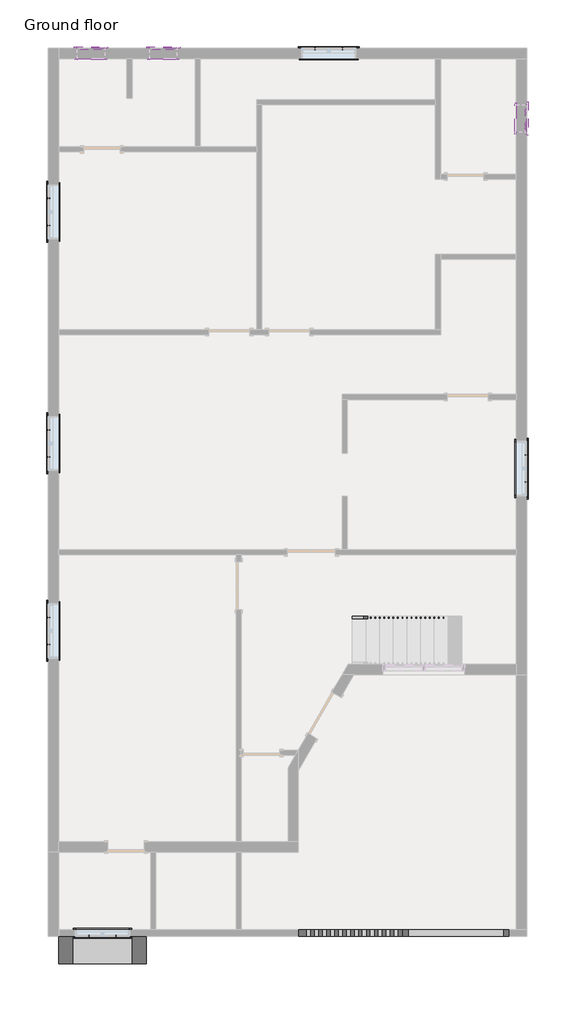
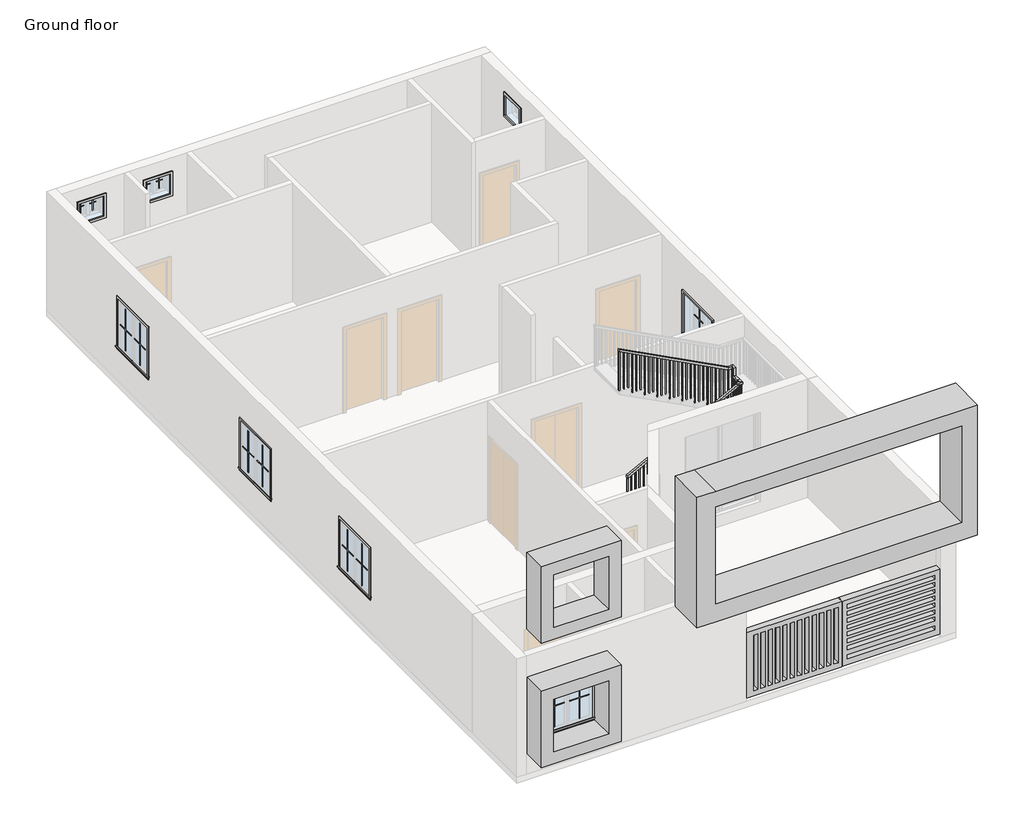
# One storey, part 3 of 3: 37 proxies, 1 railing.
"""IFC4 building model written with IfcOpenShell, lengths in millimetres."""

from ifc_helpers import new_model, si_unit, frame, origin, place, context, project, spatial, polyline, outline, extrude, faceted_brep, transform, mapped, element, save
from components import generic_models_1_generic_models_1_e6b78f1d, muntin_pattern_2x2_muntin_pattern_2x2_4dfeb3f3, muntin_pattern_2x2_muntin_pattern_2x2_e852a7e4, muntin_pattern_2x2_muntin_pattern_2x2_653c8599, muntin_pattern_2x2_muntin_pattern_2x2_c179cf80, trim_window_exterior_flat_with_sill_7cfdd449, trim_window_exterior_flat_with_sill_e6f34eb5, trim_window_interior_flat_picture_frame_f1e0b15b, trim_window_interior_flat_picture_frame_9a74d23d

model = new_model("IFC4")

# Units and contexts
model_context = context("Model", 3, world=origin())
ifc_project = project(units=[si_unit("LENGTHUNIT", "METRE", prefix="MILLI")], contexts=[model_context])

# Site, building, storey
site = spatial("IfcSite", under=ifc_project)
building = spatial("IfcBuilding", under=site)
storey = spatial("IfcBuildingStorey", under=building, Name="Ground floor", Elevation=0.0)

# Proxies
placement = place(None, origin())
generic_models_1_generic_models_1_shape = generic_models_1_generic_models_1_e6b78f1d(model_context)
element("IfcBuildingElementProxy", 1, Name="Generic Models 1 : Generic Models 1", ObjectType="Generic Models 1 : Generic Models 1", at=placement, inside=storey, context=model_context, shape_type="MappedRepresentation", body=[
    mapped(generic_models_1_generic_models_1_shape, transform((0.0, 0.0, 0.0), x_axis=(1.0, 0.0, 0.0), y_axis=(0.0, 1.0, 0.0), z_axis=(0.0, 0.0, 1.0))),
])
muntin_pattern_2x2_muntin_pattern_2x2_shape = muntin_pattern_2x2_muntin_pattern_2x2_4dfeb3f3(model_context)
element("IfcBuildingElementProxy", 2, Name="Muntin Pattern_2x2 : Muntin Pattern_2x2", ObjectType="Muntin Pattern_2x2 : Muntin Pattern_2x2", at=placement, inside=storey, context=model_context, shape_type="MappedRepresentation", body=[
    mapped(muntin_pattern_2x2_muntin_pattern_2x2_shape, transform((-5762.6039904, 6205.1114079, 984.25), x_axis=(0.0, 1.0, 0.0), y_axis=(-1.0, 0.0, 0.0), z_axis=(0.0, 0.0, 1.0))),
])
element("IfcBuildingElementProxy", 3, Name="Muntin Pattern_2x2 : Muntin Pattern_2x2", ObjectType="Muntin Pattern_2x2 : Muntin Pattern_2x2", at=placement, inside=storey, context=model_context, shape_type="MappedRepresentation", body=[
    mapped(muntin_pattern_2x2_muntin_pattern_2x2_shape, transform((-5762.6039904, 1040.9857391, 984.25), x_axis=(0.0, 1.0, 0.0), y_axis=(-1.0, 0.0, 0.0), z_axis=(0.0, 0.0, 1.0))),
])
element("IfcBuildingElementProxy", 4, Name="Muntin Pattern_2x2 : Muntin Pattern_2x2", ObjectType="Muntin Pattern_2x2 : Muntin Pattern_2x2", at=placement, inside=storey, context=model_context, shape_type="MappedRepresentation", body=[
    mapped(muntin_pattern_2x2_muntin_pattern_2x2_shape, transform((-5762.6039904, -3142.7752914, 984.25), x_axis=(0.0, 1.0, 0.0), y_axis=(-1.0, 0.0, 0.0), z_axis=(0.0, 0.0, 1.0))),
])
element("IfcBuildingElementProxy", 5, Name="Muntin Pattern_2x2 : Muntin Pattern_2x2", ObjectType="Muntin Pattern_2x2 : Muntin Pattern_2x2", at=placement, inside=storey, context=model_context, shape_type="MappedRepresentation", body=[
    mapped(muntin_pattern_2x2_muntin_pattern_2x2_shape, transform((4887.9335096, 1085.6654692, 984.25), x_axis=(0.0, -1.0, 0.0), y_axis=(1.0, 0.0, 0.0), z_axis=(0.0, 0.0, 1.0))),
])
element("IfcBuildingElementProxy", 6, Name="Muntin Pattern_2x2 : Muntin Pattern_2x2", ObjectType="Muntin Pattern_2x2 : Muntin Pattern_2x2", at=placement, inside=storey, context=model_context, shape_type="MappedRepresentation", body=[
    mapped(muntin_pattern_2x2_muntin_pattern_2x2_shape, transform((-4258.4477404, -9644.6273906, 984.25), x_axis=(-1.0, 0.0, 0.0), y_axis=(0.0, -1.0, 0.0), z_axis=(0.0, 0.0, 1.0))),
])
element("IfcBuildingElementProxy", 7, Name="Muntin Pattern_2x2 : Muntin Pattern_2x2", ObjectType="Muntin Pattern_2x2 : Muntin Pattern_2x2", at=placement, inside=storey, context=model_context, shape_type="MappedRepresentation", body=[
    mapped(muntin_pattern_2x2_muntin_pattern_2x2_shape, transform((180.9960096, 10148.3226094, 984.25), x_axis=(1.0, 0.0, 0.0), y_axis=(0.0, 1.0, 0.0), z_axis=(0.0, 0.0, 1.0))),
])
muntin_pattern_2x2_muntin_pattern_2x2_2_shape = muntin_pattern_2x2_muntin_pattern_2x2_e852a7e4(model_context)
element("IfcBuildingElementProxy", 8, Name="Muntin Pattern_2x2 : Muntin Pattern_2x2", ObjectType="Muntin Pattern_2x2 : Muntin Pattern_2x2", at=placement, inside=storey, context=model_context, shape_type="MappedRepresentation", body=[
    mapped(muntin_pattern_2x2_muntin_pattern_2x2_2_shape, transform((-5762.6039904, 6811.5364079, 984.25), x_axis=(0.0, -1.0, 0.0), y_axis=(1.0, 0.0, 0.0), z_axis=(0.0, 0.0, 1.0))),
])
element("IfcBuildingElementProxy", 9, Name="Muntin Pattern_2x2 : Muntin Pattern_2x2", ObjectType="Muntin Pattern_2x2 : Muntin Pattern_2x2", at=placement, inside=storey, context=model_context, shape_type="MappedRepresentation", body=[
    mapped(muntin_pattern_2x2_muntin_pattern_2x2_2_shape, transform((-5762.6039904, 1647.4107391, 984.25), x_axis=(0.0, -1.0, 0.0), y_axis=(1.0, 0.0, 0.0), z_axis=(0.0, 0.0, 1.0))),
])
element("IfcBuildingElementProxy", 10, Name="Muntin Pattern_2x2 : Muntin Pattern_2x2", ObjectType="Muntin Pattern_2x2 : Muntin Pattern_2x2", at=placement, inside=storey, context=model_context, shape_type="MappedRepresentation", body=[
    mapped(muntin_pattern_2x2_muntin_pattern_2x2_2_shape, transform((-5762.6039904, -2536.3502914, 984.25), x_axis=(0.0, -1.0, 0.0), y_axis=(1.0, 0.0, 0.0), z_axis=(0.0, 0.0, 1.0))),
])
element("IfcBuildingElementProxy", 11, Name="Muntin Pattern_2x2 : Muntin Pattern_2x2", ObjectType="Muntin Pattern_2x2 : Muntin Pattern_2x2", at=placement, inside=storey, context=model_context, shape_type="MappedRepresentation", body=[
    mapped(muntin_pattern_2x2_muntin_pattern_2x2_2_shape, transform((4887.9335096, 479.2404692, 984.25), x_axis=(0.0, 1.0, 0.0), y_axis=(-1.0, 0.0, 0.0), z_axis=(0.0, 0.0, 1.0))),
])
element("IfcBuildingElementProxy", 12, Name="Muntin Pattern_2x2 : Muntin Pattern_2x2", ObjectType="Muntin Pattern_2x2 : Muntin Pattern_2x2", at=placement, inside=storey, context=model_context, shape_type="MappedRepresentation", body=[
    mapped(muntin_pattern_2x2_muntin_pattern_2x2_2_shape, transform((-4864.8727404, -9644.6273906, 984.25), x_axis=(1.0, 0.0, 0.0), y_axis=(0.0, 1.0, 0.0), z_axis=(0.0, 0.0, 1.0))),
])
element("IfcBuildingElementProxy", 13, Name="Muntin Pattern_2x2 : Muntin Pattern_2x2", ObjectType="Muntin Pattern_2x2 : Muntin Pattern_2x2", at=placement, inside=storey, context=model_context, shape_type="MappedRepresentation", body=[
    mapped(muntin_pattern_2x2_muntin_pattern_2x2_2_shape, transform((787.4210096, 10148.3226094, 984.25), x_axis=(-1.0, 0.0, 0.0), y_axis=(0.0, -1.0, 0.0), z_axis=(0.0, 0.0, 1.0))),
])
muntin_pattern_2x2_muntin_pattern_2x2_3_shape = muntin_pattern_2x2_muntin_pattern_2x2_653c8599(model_context)
element("IfcBuildingElementProxy", 14, Name="Muntin Pattern_2x2 : Muntin Pattern_2x2", ObjectType="Muntin Pattern_2x2 : Muntin Pattern_2x2", at=placement, inside=storey, context=model_context, shape_type="MappedRepresentation", body=[
    mapped(muntin_pattern_2x2_muntin_pattern_2x2_3_shape, transform((-4968.4388632, 10148.3226094, 2203.45), x_axis=(1.0, 0.0, 0.0), y_axis=(0.0, 1.0, 0.0), z_axis=(0.0, 0.0, 1.0))),
])
element("IfcBuildingElementProxy", 15, Name="Muntin Pattern_2x2 : Muntin Pattern_2x2", ObjectType="Muntin Pattern_2x2 : Muntin Pattern_2x2", at=placement, inside=storey, context=model_context, shape_type="MappedRepresentation", body=[
    mapped(muntin_pattern_2x2_muntin_pattern_2x2_3_shape, transform((-3356.4344932, 10148.3226094, 2203.45), x_axis=(1.0, 0.0, 0.0), y_axis=(0.0, 1.0, 0.0), z_axis=(0.0, 0.0, 1.0))),
])
element("IfcBuildingElementProxy", 16, Name="Muntin Pattern_2x2 : Muntin Pattern_2x2", ObjectType="Muntin Pattern_2x2 : Muntin Pattern_2x2", at=placement, inside=storey, context=model_context, shape_type="MappedRepresentation", body=[
    mapped(muntin_pattern_2x2_muntin_pattern_2x2_3_shape, transform((4887.9335096, 8739.425541, 2203.45), x_axis=(0.0, -1.0, 0.0), y_axis=(1.0, 0.0, 0.0), z_axis=(0.0, 0.0, 1.0))),
])
muntin_pattern_2x2_muntin_pattern_2x2_4_shape = muntin_pattern_2x2_muntin_pattern_2x2_c179cf80(model_context)
element("IfcBuildingElementProxy", 17, Name="Muntin Pattern_2x2 : Muntin Pattern_2x2", ObjectType="Muntin Pattern_2x2 : Muntin Pattern_2x2", at=placement, inside=storey, context=model_context, shape_type="MappedRepresentation", body=[
    mapped(muntin_pattern_2x2_muntin_pattern_2x2_4_shape, transform((-4666.8138632, 10148.3226094, 2203.45), x_axis=(-1.0, 0.0, 0.0), y_axis=(0.0, -1.0, 0.0), z_axis=(0.0, 0.0, 1.0))),
])
element("IfcBuildingElementProxy", 18, Name="Muntin Pattern_2x2 : Muntin Pattern_2x2", ObjectType="Muntin Pattern_2x2 : Muntin Pattern_2x2", at=placement, inside=storey, context=model_context, shape_type="MappedRepresentation", body=[
    mapped(muntin_pattern_2x2_muntin_pattern_2x2_4_shape, transform((-3054.8094932, 10148.3226094, 2203.45), x_axis=(-1.0, 0.0, 0.0), y_axis=(0.0, -1.0, 0.0), z_axis=(0.0, 0.0, 1.0))),
])
element("IfcBuildingElementProxy", 19, Name="Muntin Pattern_2x2 : Muntin Pattern_2x2", ObjectType="Muntin Pattern_2x2 : Muntin Pattern_2x2", at=placement, inside=storey, context=model_context, shape_type="MappedRepresentation", body=[
    mapped(muntin_pattern_2x2_muntin_pattern_2x2_4_shape, transform((4887.9335096, 8437.800541, 2203.45), x_axis=(0.0, 1.0, 0.0), y_axis=(-1.0, 0.0, 0.0), z_axis=(0.0, 0.0, 1.0))),
])
trim_window_exterior_flat_with_sill_shape = trim_window_exterior_flat_with_sill_7cfdd449(model_context)
element("IfcBuildingElementProxy", 20, Name="Trim-Window-Exterior-Flat : with Sill", ObjectType="Trim-Window-Exterior-Flat : with Sill", at=placement, inside=storey, context=model_context, shape_type="MappedRepresentation", body=[
    mapped(trim_window_exterior_flat_with_sill_shape, transform((-5772.1289904, 6508.3239079, 2133.6), x_axis=(0.0, -1.0, 0.0), y_axis=(0.0, 0.0, 1.0), z_axis=(-1.0, 0.0, 0.0))),
])
element("IfcBuildingElementProxy", 21, Name="Trim-Window-Exterior-Flat : with Sill", ObjectType="Trim-Window-Exterior-Flat : with Sill", at=placement, inside=storey, context=model_context, shape_type="MappedRepresentation", body=[
    mapped(trim_window_exterior_flat_with_sill_shape, transform((-5772.1289904, 1344.1982391, 2133.6), x_axis=(0.0, -1.0, 0.0), y_axis=(0.0, 0.0, 1.0), z_axis=(-1.0, 0.0, 0.0))),
])
element("IfcBuildingElementProxy", 22, Name="Trim-Window-Exterior-Flat : with Sill", ObjectType="Trim-Window-Exterior-Flat : with Sill", at=placement, inside=storey, context=model_context, shape_type="MappedRepresentation", body=[
    mapped(trim_window_exterior_flat_with_sill_shape, transform((-5772.1289904, -2839.5627914, 2133.6), x_axis=(0.0, -1.0, 0.0), y_axis=(0.0, 0.0, 1.0), z_axis=(-1.0, 0.0, 0.0))),
])
element("IfcBuildingElementProxy", 23, Name="Trim-Window-Exterior-Flat : with Sill", ObjectType="Trim-Window-Exterior-Flat : with Sill", at=placement, inside=storey, context=model_context, shape_type="MappedRepresentation", body=[
    mapped(trim_window_exterior_flat_with_sill_shape, transform((4897.4585096, 782.4529692, 2133.6), x_axis=(0.0, 1.0, 0.0), y_axis=(0.0, 0.0, 1.0), z_axis=(1.0, 0.0, 0.0))),
])
element("IfcBuildingElementProxy", 24, Name="Trim-Window-Exterior-Flat : with Sill", ObjectType="Trim-Window-Exterior-Flat : with Sill", at=placement, inside=storey, context=model_context, shape_type="MappedRepresentation", body=[
    mapped(trim_window_exterior_flat_with_sill_shape, transform((-4561.6602404, -9654.1523906, 2133.6), x_axis=(1.0, 0.0, 0.0), y_axis=(0.0, 0.0, 1.0), z_axis=(0.0, -1.0, 0.0))),
])
element("IfcBuildingElementProxy", 25, Name="Trim-Window-Exterior-Flat : with Sill", ObjectType="Trim-Window-Exterior-Flat : with Sill", at=placement, inside=storey, context=model_context, shape_type="MappedRepresentation", body=[
    mapped(trim_window_exterior_flat_with_sill_shape, transform((484.2085096, 10157.8476094, 2133.6), x_axis=(-1.0, 0.0, 0.0), y_axis=(0.0, 0.0, 1.0), z_axis=(0.0, 1.0, 0.0))),
])
trim_window_exterior_flat_with_sill_2_shape = trim_window_exterior_flat_with_sill_e6f34eb5(model_context)
element("IfcBuildingElementProxy", 26, Name="Trim-Window-Exterior-Flat : with Sill", ObjectType="Trim-Window-Exterior-Flat : with Sill", at=placement, inside=storey, context=model_context, shape_type="MappedRepresentation", body=[
    mapped(trim_window_exterior_flat_with_sill_2_shape, transform((-4817.6263632, 10157.8476094, 2667.0), x_axis=(-1.0, 0.0, 0.0), y_axis=(0.0, 0.0, 1.0), z_axis=(0.0, 1.0, 0.0))),
])
element("IfcBuildingElementProxy", 27, Name="Trim-Window-Exterior-Flat : with Sill", ObjectType="Trim-Window-Exterior-Flat : with Sill", at=placement, inside=storey, context=model_context, shape_type="MappedRepresentation", body=[
    mapped(trim_window_exterior_flat_with_sill_2_shape, transform((-3205.6219932, 10157.8476094, 2667.0), x_axis=(-1.0, 0.0, 0.0), y_axis=(0.0, 0.0, 1.0), z_axis=(0.0, 1.0, 0.0))),
])
element("IfcBuildingElementProxy", 28, Name="Trim-Window-Exterior-Flat : with Sill", ObjectType="Trim-Window-Exterior-Flat : with Sill", at=placement, inside=storey, context=model_context, shape_type="MappedRepresentation", body=[
    mapped(trim_window_exterior_flat_with_sill_2_shape, transform((4897.4585096, 8588.613041, 2667.0), x_axis=(0.0, 1.0, 0.0), y_axis=(0.0, 0.0, 1.0), z_axis=(1.0, 0.0, 0.0))),
])
trim_window_interior_flat_picture_frame_shape = trim_window_interior_flat_picture_frame_f1e0b15b(model_context)
element("IfcBuildingElementProxy", 29, Name="Trim-Window-Interior-Flat : Picture Frame", ObjectType="Trim-Window-Interior-Flat : Picture Frame", at=placement, inside=storey, context=model_context, shape_type="MappedRepresentation", body=[
    mapped(trim_window_interior_flat_picture_frame_shape, transform((-5543.5289904, 6508.3239079, 2133.6), x_axis=(0.0, 1.0, 0.0), y_axis=(0.0, 0.0, 1.0), z_axis=(1.0, 0.0, 0.0))),
])
element("IfcBuildingElementProxy", 30, Name="Trim-Window-Interior-Flat : Picture Frame", ObjectType="Trim-Window-Interior-Flat : Picture Frame", at=placement, inside=storey, context=model_context, shape_type="MappedRepresentation", body=[
    mapped(trim_window_interior_flat_picture_frame_shape, transform((-5543.5289904, 1344.1982391, 2133.6), x_axis=(0.0, 1.0, 0.0), y_axis=(0.0, 0.0, 1.0), z_axis=(1.0, 0.0, 0.0))),
])
element("IfcBuildingElementProxy", 31, Name="Trim-Window-Interior-Flat : Picture Frame", ObjectType="Trim-Window-Interior-Flat : Picture Frame", at=placement, inside=storey, context=model_context, shape_type="MappedRepresentation", body=[
    mapped(trim_window_interior_flat_picture_frame_shape, transform((-5543.5289904, -2839.5627914, 2133.6), x_axis=(0.0, 1.0, 0.0), y_axis=(0.0, 0.0, 1.0), z_axis=(1.0, 0.0, 0.0))),
])
element("IfcBuildingElementProxy", 32, Name="Trim-Window-Interior-Flat : Picture Frame", ObjectType="Trim-Window-Interior-Flat : Picture Frame", at=placement, inside=storey, context=model_context, shape_type="MappedRepresentation", body=[
    mapped(trim_window_interior_flat_picture_frame_shape, transform((4668.8585096, 782.4529692, 2133.6), x_axis=(0.0, -1.0, 0.0), y_axis=(0.0, 0.0, 1.0), z_axis=(-1.0, 0.0, 0.0))),
])
element("IfcBuildingElementProxy", 33, Name="Trim-Window-Interior-Flat : Picture Frame", ObjectType="Trim-Window-Interior-Flat : Picture Frame", at=placement, inside=storey, context=model_context, shape_type="MappedRepresentation", body=[
    mapped(trim_window_interior_flat_picture_frame_shape, transform((-4561.6602404, -9501.7523906, 2133.6), x_axis=(-1.0, 0.0, 0.0), y_axis=(0.0, 0.0, 1.0), z_axis=(0.0, 1.0, 0.0))),
])
element("IfcBuildingElementProxy", 34, Name="Trim-Window-Interior-Flat : Picture Frame", ObjectType="Trim-Window-Interior-Flat : Picture Frame", at=placement, inside=storey, context=model_context, shape_type="MappedRepresentation", body=[
    mapped(trim_window_interior_flat_picture_frame_shape, transform((484.2085096, 9929.2476094, 2133.6), x_axis=(1.0, 0.0, 0.0), y_axis=(0.0, 0.0, 1.0), z_axis=(0.0, -1.0, 0.0))),
])
trim_window_interior_flat_picture_frame_2_shape = trim_window_interior_flat_picture_frame_9a74d23d(model_context)
element("IfcBuildingElementProxy", 35, Name="Trim-Window-Interior-Flat : Picture Frame", ObjectType="Trim-Window-Interior-Flat : Picture Frame", at=placement, inside=storey, context=model_context, shape_type="MappedRepresentation", body=[
    mapped(trim_window_interior_flat_picture_frame_2_shape, transform((-4817.6263632, 9929.2476094, 2667.0), x_axis=(1.0, 0.0, 0.0), y_axis=(0.0, 0.0, 1.0), z_axis=(0.0, -1.0, 0.0))),
])
element("IfcBuildingElementProxy", 36, Name="Trim-Window-Interior-Flat : Picture Frame", ObjectType="Trim-Window-Interior-Flat : Picture Frame", at=placement, inside=storey, context=model_context, shape_type="MappedRepresentation", body=[
    mapped(trim_window_interior_flat_picture_frame_2_shape, transform((-3205.6219932, 9929.2476094, 2667.0), x_axis=(1.0, 0.0, 0.0), y_axis=(0.0, 0.0, 1.0), z_axis=(0.0, -1.0, 0.0))),
])
element("IfcBuildingElementProxy", 37, Name="Trim-Window-Interior-Flat : Picture Frame", ObjectType="Trim-Window-Interior-Flat : Picture Frame", at=placement, inside=storey, context=model_context, shape_type="MappedRepresentation", body=[
    mapped(trim_window_interior_flat_picture_frame_2_shape, transform((4668.8585096, 8588.613041, 2667.0), x_axis=(0.0, -1.0, 0.0), y_axis=(0.0, 0.0, 1.0), z_axis=(-1.0, 0.0, 0.0))),
])

# Railing
element("IfcRailing", 38, ObjectType="Handrail - Rectangular", at=placement, inside=storey, context=model_context, shape_type="SolidModel", body=[
    faceted_brep([(1011.2585096, -2516.7523906, 1074.42), (1011.2585096, -2516.7523906, 1017.0446664), (1011.2585096, -2567.5523906, 1017.0446664), (1011.2585096, -2567.5523906, 1074.42), (3678.2585096, -2516.7523906, 2474.595), (3729.0585096, -2516.7523906, 2443.8896664), (3729.0585096, -2567.5523906, 2443.8896664), (3678.2585096, -2567.5523906, 2474.595), (3678.2585096, -2516.7523906, 2514.6), (3729.0585096, -2516.7523906, 2463.8), (3729.0585096, -2567.5523906, 2463.8), (3678.2585096, -2567.5523906, 2514.6), (3754.4585096, -2516.7523906, 2514.6), (3754.4585096, -2516.7523906, 2463.8), (3805.2585096, -2567.5523906, 2463.8), (3805.2585096, -2567.5523906, 2514.6), (3754.4585096, -2440.5523906, 2514.6), (3754.4585096, -2440.5523906, 2463.8), (3805.2585096, -2440.5523906, 2463.8), (3805.2585096, -2440.5523906, 2514.6), (3754.4585096, -2288.1523906, 2514.6), (3754.4585096, -2237.3523906, 2463.8), (3805.2585096, -2237.3523906, 2463.8), (3805.2585096, -2288.1523906, 2514.6), (3754.4585096, -2288.1523906, 2714.625), (3754.4585096, -2237.3523906, 2663.825), (3805.2585096, -2237.3523906, 2663.825), (3805.2585096, -2288.1523906, 2714.625), (3754.4585096, -2211.9523906, 2714.625), (3754.4585096, -2211.9523906, 2663.825), (3805.2585096, -2161.1523906, 2663.825), (3805.2585096, -2161.1523906, 2714.625), (3678.2585096, -2211.9523906, 2714.625), (3665.7340647, -2211.9523906, 2663.825), (3665.7340647, -2161.1523906, 2663.825), (3678.2585096, -2161.1523906, 2714.625), (1011.2585096, -2211.9523906, 4114.8), (1011.2585096, -2161.1523906, 4114.8), (1011.2585096, -2161.1523906, 4057.4246664), (1011.2585096, -2211.9523906, 4057.4246664)], [[[0, 1, 2, 3]], [[1, 0, 4, 5]], [[2, 1, 5, 6]], [[3, 2, 6, 7]], [[0, 3, 7, 4]], [[5, 4, 8, 9]], [[6, 5, 9, 10]], [[7, 6, 10, 11]], [[4, 7, 11, 8]], [[9, 8, 12, 13]], [[10, 9, 13, 14]], [[11, 10, 14, 15]], [[8, 11, 15, 12]], [[13, 12, 16, 17]], [[14, 13, 17, 18]], [[15, 14, 18, 19]], [[12, 15, 19, 16]], [[17, 16, 20, 21]], [[18, 17, 21, 22]], [[19, 18, 22, 23]], [[16, 19, 23, 20]], [[21, 20, 24, 25]], [[22, 21, 25, 26]], [[23, 22, 26, 27]], [[20, 23, 27, 24]], [[25, 24, 28, 29]], [[26, 25, 29, 30]], [[27, 26, 30, 31]], [[24, 27, 31, 28]], [[29, 28, 32, 33]], [[30, 29, 33, 34]], [[31, 30, 34, 35]], [[28, 31, 35, 32]], [[36, 37, 38, 39]], [[33, 32, 36, 39]], [[34, 33, 39, 38]], [[35, 34, 38, 37]], [[32, 35, 37, 36]]]),
    extrude(outline(polyline([(4049.0902914, 1027.1335096), (3040.38, 1027.1335096), (3040.38, 1046.1835096), (4039.0890414, 1046.1835096), (4049.0902914, 1027.1335096)])), frame((0.0, -2196.0773906, 0.0), z_axis=(0.0, 1.0, 0.0), x_axis=(0.0, 0.0, 1.0)), (0.0, 0.0, 1.0), 19.05),
    extrude(outline(polyline([(3995.7502914, 1128.7335096), (3040.38, 1128.7335096), (3040.38, 1147.7835096), (3985.7490414, 1147.7835096), (3995.7502914, 1128.7335096)])), frame((0.0, -2196.0773906, 0.0), z_axis=(0.0, 1.0, 0.0), x_axis=(0.0, 0.0, 1.0)), (0.0, 0.0, 1.0), 19.05),
    extrude(outline(polyline([(3942.4102914, 1230.3335096), (3040.38, 1230.3335096), (3040.38, 1249.3835096), (3932.4090414, 1249.3835096), (3942.4102914, 1230.3335096)])), frame((0.0, -2196.0773906, 0.0), z_axis=(0.0, 1.0, 0.0), x_axis=(0.0, 0.0, 1.0)), (0.0, 0.0, 1.0), 19.05),
    extrude(outline(polyline([(3889.0702914, 1331.9335096), (2880.36, 1331.9335096), (2880.36, 1350.9835096), (3879.0690414, 1350.9835096), (3889.0702914, 1331.9335096)])), frame((0.0, -2196.0773906, 0.0), z_axis=(0.0, 1.0, 0.0), x_axis=(0.0, 0.0, 1.0)), (0.0, 0.0, 1.0), 19.05),
    extrude(outline(polyline([(3835.7302914, 1433.5335096), (2880.36, 1433.5335096), (2880.36, 1452.5835096), (3825.7290414, 1452.5835096), (3835.7302914, 1433.5335096)])), frame((0.0, -2196.0773906, 0.0), z_axis=(0.0, 1.0, 0.0), x_axis=(0.0, 0.0, 1.0)), (0.0, 0.0, 1.0), 19.05),
    extrude(outline(polyline([(3782.3902914, 1535.1335096), (2880.36, 1535.1335096), (2880.36, 1554.1835096), (3772.3890414, 1554.1835096), (3782.3902914, 1535.1335096)])), frame((0.0, -2196.0773906, 0.0), z_axis=(0.0, 1.0, 0.0), x_axis=(0.0, 0.0, 1.0)), (0.0, 0.0, 1.0), 19.05),
    extrude(outline(polyline([(3729.0502914, 1636.7335096), (2720.34, 1636.7335096), (2720.34, 1655.7835096), (3719.0490414, 1655.7835096), (3729.0502914, 1636.7335096)])), frame((0.0, -2196.0773906, 0.0), z_axis=(0.0, 1.0, 0.0), x_axis=(0.0, 0.0, 1.0)), (0.0, 0.0, 1.0), 19.05),
    extrude(outline(polyline([(3675.7102914, 1738.3335096), (2720.34, 1738.3335096), (2720.34, 1757.3835096), (3665.7090414, 1757.3835096), (3675.7102914, 1738.3335096)])), frame((0.0, -2196.0773906, 0.0), z_axis=(0.0, 1.0, 0.0), x_axis=(0.0, 0.0, 1.0)), (0.0, 0.0, 1.0), 19.05),
    extrude(outline(polyline([(3622.3702914, 1839.9335096), (2720.34, 1839.9335096), (2720.34, 1858.9835096), (3612.3690414, 1858.9835096), (3622.3702914, 1839.9335096)])), frame((0.0, -2196.0773906, 0.0), z_axis=(0.0, 1.0, 0.0), x_axis=(0.0, 0.0, 1.0)), (0.0, 0.0, 1.0), 19.05),
    extrude(outline(polyline([(3569.0302914, 1941.5335096), (2560.32, 1941.5335096), (2560.32, 1960.5835096), (3559.0290414, 1960.5835096), (3569.0302914, 1941.5335096)])), frame((0.0, -2196.0773906, 0.0), z_axis=(0.0, 1.0, 0.0), x_axis=(0.0, 0.0, 1.0)), (0.0, 0.0, 1.0), 19.05),
    extrude(outline(polyline([(3515.6902914, 2043.1335096), (2560.32, 2043.1335096), (2560.32, 2062.1835096), (3505.6890414, 2062.1835096), (3515.6902914, 2043.1335096)])), frame((0.0, -2196.0773906, 0.0), z_axis=(0.0, 1.0, 0.0), x_axis=(0.0, 0.0, 1.0)), (0.0, 0.0, 1.0), 19.05),
    extrude(outline(polyline([(3462.3502914, 2144.7335096), (2560.32, 2144.7335096), (2560.32, 2163.7835096), (3452.3490414, 2163.7835096), (3462.3502914, 2144.7335096)])), frame((0.0, -2196.0773906, 0.0), z_axis=(0.0, 1.0, 0.0), x_axis=(0.0, 0.0, 1.0)), (0.0, 0.0, 1.0), 19.05),
    extrude(outline(polyline([(3409.0102914, 2246.3335096), (2400.3, 2246.3335096), (2400.3, 2265.3835096), (3399.0090414, 2265.3835096), (3409.0102914, 2246.3335096)])), frame((0.0, -2196.0773906, 0.0), z_axis=(0.0, 1.0, 0.0), x_axis=(0.0, 0.0, 1.0)), (0.0, 0.0, 1.0), 19.05),
    extrude(outline(polyline([(3355.6702914, 2347.9335096), (2400.3, 2347.9335096), (2400.3, 2366.9835096), (3345.6690414, 2366.9835096), (3355.6702914, 2347.9335096)])), frame((0.0, -2196.0773906, 0.0), z_axis=(0.0, 1.0, 0.0), x_axis=(0.0, 0.0, 1.0)), (0.0, 0.0, 1.0), 19.05),
    extrude(outline(polyline([(3302.3302914, 2449.5335096), (2400.3, 2449.5335096), (2400.3, 2468.5835096), (3292.3290414, 2468.5835096), (3302.3302914, 2449.5335096)])), frame((0.0, -2196.0773906, 0.0), z_axis=(0.0, 1.0, 0.0), x_axis=(0.0, 0.0, 1.0)), (0.0, 0.0, 1.0), 19.05),
    extrude(outline(polyline([(3248.9902914, 2551.1335096), (2240.28, 2551.1335096), (2240.28, 2570.1835096), (3238.9890414, 2570.1835096), (3248.9902914, 2551.1335096)])), frame((0.0, -2196.0773906, 0.0), z_axis=(0.0, 1.0, 0.0), x_axis=(0.0, 0.0, 1.0)), (0.0, 0.0, 1.0), 19.05),
    extrude(outline(polyline([(3195.6502914, 2652.7335096), (2240.28, 2652.7335096), (2240.28, 2671.7835096), (3185.6490414, 2671.7835096), (3195.6502914, 2652.7335096)])), frame((0.0, -2196.0773906, 0.0), z_axis=(0.0, 1.0, 0.0), x_axis=(0.0, 0.0, 1.0)), (0.0, 0.0, 1.0), 19.05),
    extrude(outline(polyline([(3142.3102914, 2754.3335096), (2240.28, 2754.3335096), (2240.28, 2773.3835096), (3132.3090414, 2773.3835096), (3142.3102914, 2754.3335096)])), frame((0.0, -2196.0773906, 0.0), z_axis=(0.0, 1.0, 0.0), x_axis=(0.0, 0.0, 1.0)), (0.0, 0.0, 1.0), 19.05),
    extrude(outline(polyline([(3088.9702914, 2855.9335096), (2080.26, 2855.9335096), (2080.26, 2874.9835096), (3078.9690414, 2874.9835096), (3088.9702914, 2855.9335096)])), frame((0.0, -2196.0773906, 0.0), z_axis=(0.0, 1.0, 0.0), x_axis=(0.0, 0.0, 1.0)), (0.0, 0.0, 1.0), 19.05),
    extrude(outline(polyline([(3035.6302914, 2957.5335096), (2080.26, 2957.5335096), (2080.26, 2976.5835096), (3025.6290414, 2976.5835096), (3035.6302914, 2957.5335096)])), frame((0.0, -2196.0773906, 0.0), z_axis=(0.0, 1.0, 0.0), x_axis=(0.0, 0.0, 1.0)), (0.0, 0.0, 1.0), 19.05),
    extrude(outline(polyline([(2982.2902914, 3059.1335096), (2080.26, 3059.1335096), (2080.26, 3078.1835096), (2972.2890414, 3078.1835096), (2982.2902914, 3059.1335096)])), frame((0.0, -2196.0773906, 0.0), z_axis=(0.0, 1.0, 0.0), x_axis=(0.0, 0.0, 1.0)), (0.0, 0.0, 1.0), 19.05),
    extrude(outline(polyline([(2928.9502914, 3160.7335096), (1920.24, 3160.7335096), (1920.24, 3179.7835096), (2918.9490414, 3179.7835096), (2928.9502914, 3160.7335096)])), frame((0.0, -2196.0773906, 0.0), z_axis=(0.0, 1.0, 0.0), x_axis=(0.0, 0.0, 1.0)), (0.0, 0.0, 1.0), 19.05),
    extrude(outline(polyline([(2875.6102914, 3262.3335096), (1920.24, 3262.3335096), (1920.24, 3281.3835096), (2865.6090414, 3281.3835096), (2875.6102914, 3262.3335096)])), frame((0.0, -2196.0773906, 0.0), z_axis=(0.0, 1.0, 0.0), x_axis=(0.0, 0.0, 1.0)), (0.0, 0.0, 1.0), 19.05),
    extrude(outline(polyline([(2822.2702914, 3363.9335096), (1920.24, 3363.9335096), (1920.24, 3382.9835096), (2812.2690414, 3382.9835096), (2822.2702914, 3363.9335096)])), frame((0.0, -2196.0773906, 0.0), z_axis=(0.0, 1.0, 0.0), x_axis=(0.0, 0.0, 1.0)), (0.0, 0.0, 1.0), 19.05),
    extrude(outline(polyline([(2768.9302914, 3465.5335096), (1760.22, 3465.5335096), (1760.22, 3484.5835096), (2758.9290414, 3484.5835096), (2768.9302914, 3465.5335096)])), frame((0.0, -2196.0773906, 0.0), z_axis=(0.0, 1.0, 0.0), x_axis=(0.0, 0.0, 1.0)), (0.0, 0.0, 1.0), 19.05),
    extrude(outline(polyline([(2715.5902914, 3567.1335096), (1760.22, 3567.1335096), (1760.22, 3586.1835096), (2705.5890414, 3586.1835096), (2715.5902914, 3567.1335096)])), frame((0.0, -2196.0773906, 0.0), z_axis=(0.0, 1.0, 0.0), x_axis=(0.0, 0.0, 1.0)), (0.0, 0.0, 1.0), 19.05),
    extrude(outline(polyline([(2662.2502914, 3668.7335096), (1760.22, 3668.7335096), (1760.22, 3687.7835096), (2652.2490414, 3687.7835096), (2662.2502914, 3668.7335096)])), frame((0.0, -2196.0773906, 0.0), z_axis=(0.0, 1.0, 0.0), x_axis=(0.0, 0.0, 1.0)), (0.0, 0.0, 1.0), 19.05),
    extrude(outline(polyline([(3770.3335096, -2246.8773906), (3770.3335096, -2227.8273906), (3789.3835096, -2227.8273906), (3789.3835096, -2246.8773906), (3770.3335096, -2246.8773906)])), frame((0.0, 0.0, 1600.2), z_axis=(0.0, 0.0, 1.0), x_axis=(1.0, 0.0, 0.0)), (0.0, 0.0, 1.0), 1063.625),
    extrude(outline(polyline([(3770.3335096, -2348.4773906), (3770.3335096, -2329.4273906), (3789.3835096, -2329.4273906), (3789.3835096, -2348.4773906), (3770.3335096, -2348.4773906)])), frame((0.0, 0.0, 1600.2), z_axis=(0.0, 0.0, 1.0), x_axis=(1.0, 0.0, 0.0)), (0.0, 0.0, 1.0), 863.6),
    extrude(outline(polyline([(3770.3335096, -2450.0773906), (3770.3335096, -2431.0273906), (3789.3835096, -2431.0273906), (3789.3835096, -2450.0773906), (3770.3335096, -2450.0773906)])), frame((0.0, 0.0, 1600.2), z_axis=(0.0, 0.0, 1.0), x_axis=(1.0, 0.0, 0.0)), (0.0, 0.0, 1.0), 863.6),
    extrude(outline(polyline([(3744.9335096, -2532.6273906), (3763.9835096, -2532.6273906), (3763.9835096, -2551.6773906), (3744.9335096, -2551.6773906), (3744.9335096, -2532.6273906)])), frame((0.0, 0.0, 1600.2), z_axis=(0.0, 0.0, 1.0), x_axis=(1.0, 0.0, 0.0)), (0.0, 0.0, 1.0), 863.6),
    extrude(outline(polyline([(2398.8840414, 3643.3335096), (1440.18, 3643.3335096), (1440.18, 3662.3835096), (2408.8852914, 3662.3835096), (2398.8840414, 3643.3335096)])), frame((0.0, -2551.6773906, 0.0), z_axis=(0.0, 1.0, 0.0), x_axis=(0.0, 0.0, 1.0)), (0.0, 0.0, 1.0), 19.05),
    extrude(outline(polyline([(2345.5440414, 3541.7335096), (1440.18, 3541.7335096), (1440.18, 3560.7835096), (2355.5452914, 3560.7835096), (2345.5440414, 3541.7335096)])), frame((0.0, -2551.6773906, 0.0), z_axis=(0.0, 1.0, 0.0), x_axis=(0.0, 0.0, 1.0)), (0.0, 0.0, 1.0), 19.05),
    extrude(outline(polyline([(2292.2040414, 3440.1335096), (1440.18, 3440.1335096), (1440.18, 3459.1835096), (2302.2052914, 3459.1835096), (2292.2040414, 3440.1335096)])), frame((0.0, -2551.6773906, 0.0), z_axis=(0.0, 1.0, 0.0), x_axis=(0.0, 0.0, 1.0)), (0.0, 0.0, 1.0), 19.05),
    extrude(outline(polyline([(2238.8640414, 3338.5335096), (1280.16, 3338.5335096), (1280.16, 3357.5835096), (2248.8652914, 3357.5835096), (2238.8640414, 3338.5335096)])), frame((0.0, -2551.6773906, 0.0), z_axis=(0.0, 1.0, 0.0), x_axis=(0.0, 0.0, 1.0)), (0.0, 0.0, 1.0), 19.05),
    extrude(outline(polyline([(2185.5240414, 3236.9335096), (1280.16, 3236.9335096), (1280.16, 3255.9835096), (2195.5252914, 3255.9835096), (2185.5240414, 3236.9335096)])), frame((0.0, -2551.6773906, 0.0), z_axis=(0.0, 1.0, 0.0), x_axis=(0.0, 0.0, 1.0)), (0.0, 0.0, 1.0), 19.05),
    extrude(outline(polyline([(2132.1840414, 3135.3335096), (1280.16, 3135.3335096), (1280.16, 3154.3835096), (2142.1852914, 3154.3835096), (2132.1840414, 3135.3335096)])), frame((0.0, -2551.6773906, 0.0), z_axis=(0.0, 1.0, 0.0), x_axis=(0.0, 0.0, 1.0)), (0.0, 0.0, 1.0), 19.05),
    extrude(outline(polyline([(2078.8440414, 3033.7335096), (1120.14, 3033.7335096), (1120.14, 3052.7835096), (2088.8452914, 3052.7835096), (2078.8440414, 3033.7335096)])), frame((0.0, -2551.6773906, 0.0), z_axis=(0.0, 1.0, 0.0), x_axis=(0.0, 0.0, 1.0)), (0.0, 0.0, 1.0), 19.05),
    extrude(outline(polyline([(2025.5040414, 2932.1335096), (1120.14, 2932.1335096), (1120.14, 2951.1835096), (2035.5052914, 2951.1835096), (2025.5040414, 2932.1335096)])), frame((0.0, -2551.6773906, 0.0), z_axis=(0.0, 1.0, 0.0), x_axis=(0.0, 0.0, 1.0)), (0.0, 0.0, 1.0), 19.05),
    extrude(outline(polyline([(1972.1640414, 2830.5335096), (1120.14, 2830.5335096), (1120.14, 2849.5835096), (1982.1652914, 2849.5835096), (1972.1640414, 2830.5335096)])), frame((0.0, -2551.6773906, 0.0), z_axis=(0.0, 1.0, 0.0), x_axis=(0.0, 0.0, 1.0)), (0.0, 0.0, 1.0), 19.05),
    extrude(outline(polyline([(1918.8240414, 2728.9335096), (960.12, 2728.9335096), (960.12, 2747.9835096), (1928.8252914, 2747.9835096), (1918.8240414, 2728.9335096)])), frame((0.0, -2551.6773906, 0.0), z_axis=(0.0, 1.0, 0.0), x_axis=(0.0, 0.0, 1.0)), (0.0, 0.0, 1.0), 19.05),
    extrude(outline(polyline([(1865.4840414, 2627.3335096), (960.12, 2627.3335096), (960.12, 2646.3835096), (1875.4852914, 2646.3835096), (1865.4840414, 2627.3335096)])), frame((0.0, -2551.6773906, 0.0), z_axis=(0.0, 1.0, 0.0), x_axis=(0.0, 0.0, 1.0)), (0.0, 0.0, 1.0), 19.05),
    extrude(outline(polyline([(1812.1440414, 2525.7335096), (960.12, 2525.7335096), (960.12, 2544.7835096), (1822.1452914, 2544.7835096), (1812.1440414, 2525.7335096)])), frame((0.0, -2551.6773906, 0.0), z_axis=(0.0, 1.0, 0.0), x_axis=(0.0, 0.0, 1.0)), (0.0, 0.0, 1.0), 19.05),
    extrude(outline(polyline([(1758.8040414, 2424.1335096), (800.1, 2424.1335096), (800.1, 2443.1835096), (1768.8052914, 2443.1835096), (1758.8040414, 2424.1335096)])), frame((0.0, -2551.6773906, 0.0), z_axis=(0.0, 1.0, 0.0), x_axis=(0.0, 0.0, 1.0)), (0.0, 0.0, 1.0), 19.05),
    extrude(outline(polyline([(1705.4640414, 2322.5335096), (800.1, 2322.5335096), (800.1, 2341.5835096), (1715.4652914, 2341.5835096), (1705.4640414, 2322.5335096)])), frame((0.0, -2551.6773906, 0.0), z_axis=(0.0, 1.0, 0.0), x_axis=(0.0, 0.0, 1.0)), (0.0, 0.0, 1.0), 19.05),
    extrude(outline(polyline([(1652.1240414, 2220.9335096), (800.1, 2220.9335096), (800.1, 2239.9835096), (1662.1252914, 2239.9835096), (1652.1240414, 2220.9335096)])), frame((0.0, -2551.6773906, 0.0), z_axis=(0.0, 1.0, 0.0), x_axis=(0.0, 0.0, 1.0)), (0.0, 0.0, 1.0), 19.05),
    extrude(outline(polyline([(1598.7840414, 2119.3335096), (640.08, 2119.3335096), (640.08, 2138.3835096), (1608.7852914, 2138.3835096), (1598.7840414, 2119.3335096)])), frame((0.0, -2551.6773906, 0.0), z_axis=(0.0, 1.0, 0.0), x_axis=(0.0, 0.0, 1.0)), (0.0, 0.0, 1.0), 19.05),
    extrude(outline(polyline([(1545.4440414, 2017.7335096), (640.08, 2017.7335096), (640.08, 2036.7835096), (1555.4452914, 2036.7835096), (1545.4440414, 2017.7335096)])), frame((0.0, -2551.6773906, 0.0), z_axis=(0.0, 1.0, 0.0), x_axis=(0.0, 0.0, 1.0)), (0.0, 0.0, 1.0), 19.05),
    extrude(outline(polyline([(1492.1040414, 1916.1335096), (640.08, 1916.1335096), (640.08, 1935.1835096), (1502.1052914, 1935.1835096), (1492.1040414, 1916.1335096)])), frame((0.0, -2551.6773906, 0.0), z_axis=(0.0, 1.0, 0.0), x_axis=(0.0, 0.0, 1.0)), (0.0, 0.0, 1.0), 19.05),
    extrude(outline(polyline([(1438.7640414, 1814.5335096), (480.06, 1814.5335096), (480.06, 1833.5835096), (1448.7652914, 1833.5835096), (1438.7640414, 1814.5335096)])), frame((0.0, -2551.6773906, 0.0), z_axis=(0.0, 1.0, 0.0), x_axis=(0.0, 0.0, 1.0)), (0.0, 0.0, 1.0), 19.05),
    extrude(outline(polyline([(1385.4240414, 1712.9335096), (480.06, 1712.9335096), (480.06, 1731.9835096), (1395.4252914, 1731.9835096), (1385.4240414, 1712.9335096)])), frame((0.0, -2551.6773906, 0.0), z_axis=(0.0, 1.0, 0.0), x_axis=(0.0, 0.0, 1.0)), (0.0, 0.0, 1.0), 19.05),
    extrude(outline(polyline([(1332.0840414, 1611.3335096), (480.06, 1611.3335096), (480.06, 1630.3835096), (1342.0852914, 1630.3835096), (1332.0840414, 1611.3335096)])), frame((0.0, -2551.6773906, 0.0), z_axis=(0.0, 1.0, 0.0), x_axis=(0.0, 0.0, 1.0)), (0.0, 0.0, 1.0), 19.05),
    extrude(outline(polyline([(1278.7440414, 1509.7335096), (320.04, 1509.7335096), (320.04, 1528.7835096), (1288.7452914, 1528.7835096), (1278.7440414, 1509.7335096)])), frame((0.0, -2551.6773906, 0.0), z_axis=(0.0, 1.0, 0.0), x_axis=(0.0, 0.0, 1.0)), (0.0, 0.0, 1.0), 19.05),
    extrude(outline(polyline([(1225.4040414, 1408.1335096), (320.04, 1408.1335096), (320.04, 1427.1835096), (1235.4052914, 1427.1835096), (1225.4040414, 1408.1335096)])), frame((0.0, -2551.6773906, 0.0), z_axis=(0.0, 1.0, 0.0), x_axis=(0.0, 0.0, 1.0)), (0.0, 0.0, 1.0), 19.05),
    extrude(outline(polyline([(1172.0640414, 1306.5335096), (320.04, 1306.5335096), (320.04, 1325.5835096), (1182.0652914, 1325.5835096), (1172.0640414, 1306.5335096)])), frame((0.0, -2551.6773906, 0.0), z_axis=(0.0, 1.0, 0.0), x_axis=(0.0, 0.0, 1.0)), (0.0, 0.0, 1.0), 19.05),
    extrude(outline(polyline([(1118.7240414, 1204.9335096), (160.02, 1204.9335096), (160.02, 1223.9835096), (1128.7252914, 1223.9835096), (1118.7240414, 1204.9335096)])), frame((0.0, -2551.6773906, 0.0), z_axis=(0.0, 1.0, 0.0), x_axis=(0.0, 0.0, 1.0)), (0.0, 0.0, 1.0), 19.05),
    extrude(outline(polyline([(1065.3840414, 1103.3335096), (160.02, 1103.3335096), (160.02, 1122.3835096), (1075.3852914, 1122.3835096), (1065.3840414, 1103.3335096)])), frame((0.0, -2551.6773906, 0.0), z_axis=(0.0, 1.0, 0.0), x_axis=(0.0, 0.0, 1.0)), (0.0, 0.0, 1.0), 19.05),
    extrude(outline(polyline([(3770.3335096, -2196.0773906), (3770.3335096, -2177.0273906), (3789.3835096, -2177.0273906), (3789.3835096, -2196.0773906), (3770.3335096, -2196.0773906)])), frame((0.0, 0.0, 1600.2), z_axis=(0.0, 0.0, 1.0), x_axis=(1.0, 0.0, 0.0)), (0.0, 0.0, 1.0), 1063.625),
    extrude(outline(polyline([(3770.3335096, -2532.6273906), (3789.3835096, -2532.6273906), (3789.3835096, -2551.6773906), (3770.3335096, -2551.6773906), (3770.3335096, -2532.6273906)])), frame((0.0, 0.0, 1600.2), z_axis=(0.0, 0.0, 1.0), x_axis=(1.0, 0.0, 0.0)), (0.0, 0.0, 1.0), 863.6),
    extrude(outline(polyline([(4057.4246664, 1011.2585096), (3040.38, 1011.2585096), (3040.38, 1030.3085096), (4047.4234164, 1030.3085096), (4057.4246664, 1011.2585096)])), frame((0.0, -2196.0773906, 0.0), z_axis=(0.0, 1.0, 0.0), x_axis=(0.0, 0.0, 1.0)), (0.0, 0.0, 1.0), 19.05),
    extrude(outline(polyline([(1017.0446664, 1011.2585096), (160.02, 1011.2585096), (160.02, 1030.3085096), (1027.0459164, 1030.3085096), (1017.0446664, 1011.2585096)])), frame((0.0, -2551.6773906, 0.0), z_axis=(0.0, 1.0, 0.0), x_axis=(0.0, 0.0, 1.0)), (0.0, 0.0, 1.0), 19.05),
])

save(model, "model.ifc")

# Revit data of these elements
# Type "Muntin Pattern_2x2 : Muntin Pattern_2x2"
#   Width [instance default] = 4' - 0"
#   Thickness = 0' - 0 1/2"
#   Height [instance default] = 4' - 0"
#   Distance = 0' - 0 3/4"
#   Interior Material [instance default] = none
#   Exterior Material [instance default] = none
#   Default Elevation = 0
# Type "Trim-Window-Exterior-Flat : with Sill"
#   Trim Width = 0' - 2 1/4"
#   Trim Thickness_Picture Frame = 0' - 1 1/4"
#   Trim Thickness_with Sill = 0' - 0 3/4"
#   Sill Thickness = 0' - 1 1/4"
#   Opening Width [instance default] = 2' - 0"
#   Opening Height [instance default] = 3' - 0"
#   Default Elevation = 4' - 0"
#   Sill = yes
#   Picture Frame = no
#   Trim Material [instance default] = none
# Type "Trim-Window-Interior-Flat : Picture Frame"
#   Trim Thickness_Picture Frame = 0' - 1 1/4"
#   Trim Width = 0' - 2 1/4"
#   Trim Thickness_with Sill = 0' - 0 3/4"
#   Sill Thickness = 0' - 1 1/4"
#   Opening Width [instance default] = 2' - 0"
#   Opening Height [instance default] = 3' - 0"
#   Default Elevation = 4' - 0"
#   Sill = no
#   Picture Frame = yes
#   Trim Material [instance default] = none
# Type "Handrail - Rectangular"
#   Assembly Code = "C2010400"
#   built-in parameter 1008612 = 0.0416667 (stored number, unit not read)
#   built-in parameter 1008611 = 0.0416667 (stored number, unit not read)
#   built-in parameter 1008609 = 0.333333 (stored number, unit not read)
#   built-in parameter 1008604 = 0.166667 (stored number, unit not read)
#   built-in parameter 1008603 = 0.166667 (stored number, unit not read)
#   Railing Height = 3' - 0"
#   built-in parameter 1008630 = 2
#   built-in parameter 1008610 = 2
#   built-in parameter 1008618 = Baluster - Square : 3/4"
# Element 1 (IfcBuildingElementProxy, "Generic Models 1 : Generic Models 1")
#   Phase Created = New Construction
#   Materials on its faces: "Wood Planks", "wood 1"
# Elements 2, 3, 4, 5, 6, 7, 8, 9, 10, 11, 12, 13 (IfcBuildingElementProxy, "Muntin Pattern_2x2 : Muntin Pattern_2x2")
#   Width = 1' - 6 5/8"
#   Height = 3' - 6 1/2"
#   Interior Material = Wood - Stained
#   Exterior Material = Clad - White
#   Phase Created = New Construction
#   Materials on its faces: "Clad - White", "Wood - Stained"
# Elements 14, 15, 16, 17, 18, 19 (IfcBuildingElementProxy, "Muntin Pattern_2x2 : Muntin Pattern_2x2")
#   Width = 0' - 6 5/8"
#   Height = 1' - 3 1/2"
#   Interior Material = Wood - Stained
#   Exterior Material = Clad - White
#   Phase Created = New Construction
#   Materials on its faces: "Clad - White", "Wood - Stained"
# Elements 20, 21, 22, 23, 24, 25 (IfcBuildingElementProxy, "Trim-Window-Exterior-Flat : with Sill")
#   Opening Width = 4' - 0"
#   Opening Height = 4' - 0"
#   Trim Material = Clad - White
#   Phase Created = New Construction
#   Materials on its faces: "Clad - White"
# Elements 26, 27, 28 (IfcBuildingElementProxy, "Trim-Window-Exterior-Flat : with Sill")
#   Opening Width = 2' - 0"
#   Opening Height = 1' - 9"
#   Trim Material = Clad - White
#   Phase Created = New Construction
#   Materials on its faces: "Clad - White"
# Elements 29, 30, 31, 32, 33, 34 (IfcBuildingElementProxy, "Trim-Window-Interior-Flat : Picture Frame")
#   Opening Width = 4' - 0"
#   Opening Height = 4' - 0"
#   Trim Material = Wood - Stained
#   Phase Created = New Construction
#   Materials on its faces: "Wood - Stained"
# Elements 35, 36, 37 (IfcBuildingElementProxy, "Trim-Window-Interior-Flat : Picture Frame")
#   Opening Width = 2' - 0"
#   Opening Height = 1' - 9"
#   Trim Material = Wood - Stained
#   Phase Created = New Construction
#   Materials on its faces: "Wood - Stained"
# Element 38 (IfcRailing, "Handrail - Rectangular")
#   Phase Created = New Construction
# Materials
#   "Wood Planks": class "Wood", colour RGB 193 160 115, transparency 0, Description = "Physical material.", Cost = 0
#   "wood 1": class "Generic", colour RGB 51 32 15, transparency 0, Cost = 0
#   "Clad - White": class "Wood", colour RGB 242 242 238, transparency 0, Cost = 0
#   "Wood - Stained": class "Wood", colour RGB 224 178 126, transparency 0, Cost = 0
